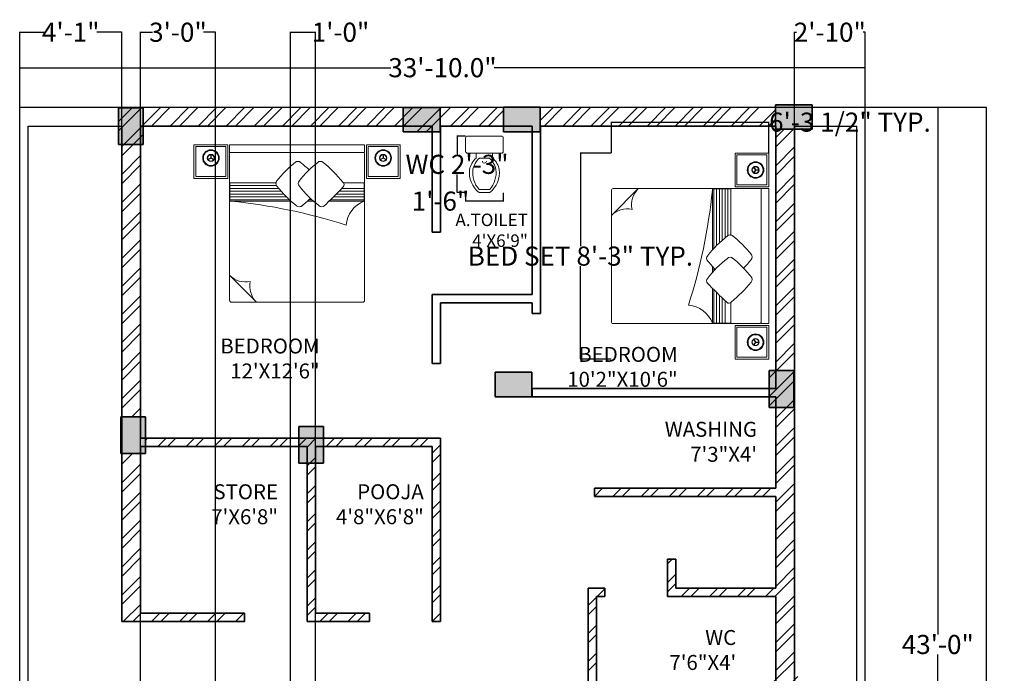
# Model space of a CAD drawing. Units: inches. Extents: x 104 to 629, y 1868 to 5138.
# Tile 2 of 2: x 156 to 629, y 2309 to 2623. Entities that reach past the tile are written whole.
import ezdxf

# ---------------------------------------------------------------- set-up
doc = ezdxf.new("R2010")
doc.units = ezdxf.units.IN
for name, color, linetype, lineweight in [('00 FURNITURE', 15, 'Continuous', 15), ('A-ANNO-DIMS', 2, 'Continuous', 18), ('A-AREA-IDEN', 7, 'Continuous', 18), ('A-FLOR-FIXT', 9, 'Continuous', 18), ('A-WALL-PATT', 8, 'Continuous', 13), ('C-PROP', 7, 'Continuous', 25), ('column', 10, 'Continuous', 35), ('hatch column', 10, 'Continuous', 13), ('WALL', 7, 'Continuous', 35)]:
    doc.layers.add(name, color=color, linetype=linetype, lineweight=lineweight)
doc.styles.get("Standard").update_dxf_attribs({"font": 'arial.ttf'})
doc.dimstyles.get("Standard").update_dxf_attribs({"dimtxt": 9.18, "dimasz": 0.18, "dimexe": 0.18, "dimexo": 0.0625, "dimgap": 0.09, "dimtad": 0, "dimtih": 1, "dimtoh": 1, "dimdec": 1, "dimzin": 0, "dimdsep": 46, "dimlunit": 3, "dimtxsty": 'Standard', "dimcen": 0.09, "dimadec": 0, "dimazin": 0, "dimtfac": 1, "dimtdec": 1, "dimtofl": 0, "dimtmove": 0, "dimatfit": 3, "dimfxl": 1, "dimtolj": 1, "dimtzin": 0, "dimarcsym": 0})

# ---------------------------------------------------------------- blocks, each defined once
blk = doc.blocks.new('column')
at = {"layer": 'column'}
for p, q in [((661.29, 2690.99), (673.05, 2690.99)), ((661.29, 2673.35), (661.29, 2690.99)), ((673.05, 2690.99), (673.05, 2673.35)), ((673.05, 2673.35), (661.29, 2673.35))]:
    blk.add_line(p, q, dxfattribs=at)
blk = doc.blocks.new('RGWTG')
at = {"layer": '00 FURNITURE'}
for p, q in [((578.23, 3473.51), (577.36, 3475.01)), ((578.36, 3473.58), (577.49, 3475.09)), ((578.23, 3473.58), (577.36, 3472.08)), ((578.36, 3473.51), (577.49, 3472)), ((578.29, 3473.62), (580.03, 3473.62)), ((578.29, 3473.47), (580.03, 3473.47)), ((521.93, 3464.58), (509.03, 3451.68)), ((509.03, 3422.63), (509.03, 3463.68)), ((509.93, 3464.58), (566.4, 3464.58)), ((557.53, 3463.84), (557.53, 3464.49)), ((557.53, 3464.49), (566.4, 3464.49)), ((558.2, 3464.49), (558.2, 3435.82)), ((559.57, 3464.49), (559.57, 3437.25)), ((560.94, 3464.49), (560.94, 3438.58)), ((562.3, 3464.49), (562.3, 3439.83)), ((563.67, 3464.49), (563.67, 3440.99)), ((565.04, 3464.49), (565.04, 3442.08)), ((566.4, 3464.58), (580.98, 3464.58)), ((566.4, 3464.49), (566.4, 3442.08)), ((566.4, 3464.49), (566.4, 3463.84)), ((580.98, 3464.58), (580.98, 3416.72)), ((558.2, 3426.48), (558.2, 3425.04)), ((509.03, 3400.68), (509.03, 3422.63)), ((558.2, 3416.13), (558.2, 3399.95)), ((559.57, 3414.75), (559.57, 3399.95)), ((580.98, 3416.72), (580.98, 3400.68)), ((560.94, 3413.39), (560.94, 3399.95)), ((562.3, 3412.04), (562.3, 3399.95)), ((563.67, 3410.72), (563.67, 3399.95)), ((580.08, 3399.78), (509.93, 3399.78)), ((557.53, 3399.95), (557.53, 3400.6)), ((566.4, 3399.95), (557.53, 3399.95)), ((566.4, 3400.6), (566.4, 3399.95)), ((578.23, 3390.78), (577.36, 3392.29)), ((578.23, 3390.86), (577.36, 3389.36)), ((578.36, 3390.86), (577.49, 3392.36)), ((578.36, 3390.78), (577.49, 3389.28)), ((578.29, 3390.9), (580.03, 3390.9)), ((578.29, 3390.74), (580.03, 3390.74))]:
    blk.add_line(p, q, dxfattribs=at)
for points in [[(568.43, 3465.48), (584.63, 3465.48), (584.63, 3481.68), (568.43, 3481.68)], [(569.33, 3466.38), (583.73, 3466.38), (583.73, 3480.78), (569.33, 3480.78)], [(580.98, 3399.78), (584.63, 3399.78), (584.63, 3464.58), (580.98, 3464.58)], [(568.43, 3398.88), (584.63, 3398.88), (584.63, 3382.68), (568.43, 3382.68)], [(569.33, 3397.98), (583.73, 3397.98), (583.73, 3383.58), (569.33, 3383.58)]]:
    blk.add_lwpolyline(points, close=True, dxfattribs=at)
for points in [[(566.52, 3464.49), (557.53, 3464.49), (557.53, 3435.08)], [(557.53, 3427.21), (557.53, 3424.3)], [(557.53, 3416.82), (557.53, 3399.95), (566.4, 3399.95), (566.4, 3409.94)]]:
    blk.add_lwpolyline(points, dxfattribs=at)
for centre, radius in [((578.29, 3473.54), 3.97), ((578.29, 3473.54), 3.63), ((578.29, 3473.54), 1.74), ((578.29, 3473.54), 1.56), ((578.29, 3390.82), 3.97), ((578.29, 3390.82), 3.63), ((578.29, 3390.82), 1.74), ((578.29, 3390.82), 1.56)]:
    blk.add_circle(centre, radius, dxfattribs=at)
for centre, radius, start, end in [((509.93, 3463.68), 0.9, 90, 180), ((529.65, 3456.88), 10.9, 135.0361, 191.9278), ((290.56, 3490.52), 268.3, 342.2214, 354.2925), ((516.73, 3443.97), 10.9, 78.0722, 134.9639), ((566.05, 3440.57), 1.82, 45, 135), ((533.58, 3399.31), 54.32, 37.931, 52.069), ((598.15, 3399.01), 54.32, 127.931, 142.069), ((574.84, 3431.77), 1.82, 315, 45), ((556.59, 3431.11), 1.82, 135, 225), ((597.87, 3463.6), 54.32, 217.931, 224.141), ((598.15, 3388.23), 54.32, 127.931, 142.069), ((566.05, 3429.78), 1.82, 45, 135), ((533.58, 3388.53), 54.32, 37.931, 52.069), ((533.28, 3463.88), 54.32, 316.32, 322.069), ((556.59, 3420.33), 1.82, 135, 225), ((765.33, 3619.75), 290.45, 223.6069, 226.2326), ((533.28, 3453.1), 54.32, 307.931, 322.069), ((574.84, 3420.99), 1.82, 315, 45), ((565.44, 3411.05), 1.47, 225.9674, 326.8337), ((545.02, 3395.29), 13.35, 20.4224, 85.5825), ((509.93, 3400.68), 0.9, 180, 270), ((580.08, 3400.68), 0.9, 270, 0)]:
    blk.add_arc(centre, radius, start, end, dxfattribs=at)
blk = doc.blocks.new('A$C2AC94788')
for p, q in [((0, 0.505), (0, 0.665)), ((0.025, 0.69), (0.435, 0.69)), ((0.46, 0.665), (0.46, 0.505)), ((0.435, 0.48), (0.025, 0.48)), ((0.13, 0.48), (0.13, 0.42)), ((0.17, 0.42), (0.29, 0.42)), ((0.33, 0.42), (0.33, 0.48)), ((0.164, 0.039), (0.296, 0.039)), ((0.229, 0.039), (0.23, 0.039)), ((0.231, 0.039), (0.23, 0.039)), ((0.165, 0), (0.295, 0))]:
    blk.add_line(p, q)
for centre, radius, start, end in [((0.025, 0.665), 0.025, 90, 180), ((0.435, 0.665), 0.025, 0, 90), ((0.025, 0.505), 0.025, 180, 270), ((0.435, 0.505), 0.025, 270, 0), ((0.287, 0.236), 0.242, 130.4885, 169.445), ((0.327, 0.236), 0.242, 130.4885, 169.445), ((0.23, 0.385), 0.025, 180, 0), ((0.133, 0.236), 0.242, 10.555, 49.5115), ((0.173, 0.236), 0.242, 10.555, 49.5115), ((0.36, 0.245), 0.313, 173.5369, 231.4483), ((0.4, 0.245), 0.313, 173.5369, 221.0604), ((0.1, 0.245), 0.313, 308.5517, 6.4631), ((0.06, 0.245), 0.313, 318.9396, 6.4631)]:
    blk.add_arc(centre, radius, start, end)
blk = doc.blocks.new('*D13')
at = {"layer": 'A-ANNO-DIMS', "color": 0, "lineweight": -2, "transparency": 16777216}
for p, q in [((155.91, 2581.05), (155.91, 2600.18)), ((156.09, 2600), (334.14, 2600)), ((561.73, 2600), (383.68, 2600)), ((561.91, 2581.05), (561.91, 2600.18))]:
    blk.add_line(p, q, dxfattribs=at)
at = {"layer": 'A-ANNO-DIMS', "color": 0, "transparency": 16777216}
for points in [[(156.09, 2600.03), (156.09, 2599.97), (155.91, 2600)], [(561.73, 2600.03), (561.73, 2599.97), (561.91, 2600)]]:
    blk.add_solid(points, dxfattribs=at)
at = {"layer": 'Defpoints', "color": 0, "transparency": 16777216}
for p in [(561.91, 2600), (155.91, 2580.99), (561.91, 2580.99)]:
    blk.add_point(p, dxfattribs=at)
at = {"layer": 'A-ANNO-DIMS', "color": 0, "transparency": 16777216, "insert": (358.91, 2600), "char_height": 9.18, "attachment_point": 5}
blk.add_mtext('\\A1;33\'-10.0"', dxfattribs=at)
blk = doc.blocks.new('*D14')
at = {"layer": 'A-ANNO-DIMS', "color": 0, "lineweight": -2, "transparency": 16777216}
for p, q in [((561.97, 2580.99), (620.18, 2580.99)), ((620, 2580.81), (620, 2249.77)), ((620, 1909.17), (620, 2240.21)), ((561.97, 1908.99), (620.18, 1908.99))]:
    blk.add_line(p, q, dxfattribs=at)
at = {"layer": 'A-ANNO-DIMS', "color": 0, "transparency": 16777216}
for points in [[(619.97, 2580.81), (620.03, 2580.81), (620, 2580.99)], [(619.97, 1909.17), (620.03, 1909.17), (620, 1908.99)]]:
    blk.add_solid(points, dxfattribs=at)
at = {"layer": 'Defpoints', "color": 0, "transparency": 16777216}
for p in [(561.91, 2580.99), (561.91, 1908.99), (620, 1908.99)]:
    blk.add_point(p, dxfattribs=at)
at = {"layer": 'A-ANNO-DIMS', "color": 0, "transparency": 16777216, "insert": (620, 2244.99), "char_height": 9.18, "attachment_point": 5}
blk.add_mtext("\\A1;56'", dxfattribs=at)
blk = doc.blocks.new('*D17')
at = {"layer": 'A-ANNO-DIMS', "color": 0, "lineweight": -2, "transparency": 16777216}
for p, q in [((439.94, 2559), (424.97, 2559)), ((425.15, 2558.82), (425.15, 2514.34)), ((425.15, 2460.18), (425.15, 2504.66)), ((439.94, 2460), (424.97, 2460))]:
    blk.add_line(p, q, dxfattribs=at)
at = {"layer": 'A-ANNO-DIMS', "color": 0, "transparency": 16777216}
for points in [[(425.12, 2558.82), (425.18, 2558.82), (425.15, 2559)], [(425.12, 2460.18), (425.18, 2460.18), (425.15, 2460)]]:
    blk.add_solid(points, dxfattribs=at)
at = {"layer": 'Defpoints', "color": 0, "transparency": 16777216}
for p in [(425.15, 2559), (440, 2559), (440, 2460)]:
    blk.add_point(p, dxfattribs=at)
at = {"layer": 'A-ANNO-DIMS', "color": 0, "transparency": 16777216, "insert": (425.15, 2509.5), "char_height": 9.18, "attachment_point": 5}
blk.add_mtext('\\A1;BED SET 8\'-3" TYP.', dxfattribs=at)
blk = doc.blocks.new('*D18')
at = {"layer": 'A-ANNO-DIMS', "color": 0, "lineweight": -2, "transparency": 16777216}
for p, q in [((440, 2559.06), (440, 2574.03)), ((440.18, 2573.85), (515.42, 2573.85)), ((515.6, 2559.06), (515.6, 2574.03)), ((515.6, 2573.85), (515.78, 2573.85))]:
    blk.add_line(p, q, dxfattribs=at)
at = {"layer": 'A-ANNO-DIMS', "color": 0, "transparency": 16777216}
for points in [[(440.18, 2573.88), (440.18, 2573.82), (440, 2573.85)], [(515.42, 2573.88), (515.42, 2573.82), (515.6, 2573.85)]]:
    blk.add_solid(points, dxfattribs=at)
at = {"layer": 'Defpoints', "color": 0, "transparency": 16777216}
for p in [(515.6, 2573.85), (440, 2559), (515.6, 2559)]:
    blk.add_point(p, dxfattribs=at)
at = {"layer": 'A-ANNO-DIMS', "color": 0, "transparency": 16777216, "insert": (554.57, 2573.85), "char_height": 9.18, "attachment_point": 5}
blk.add_mtext('\\A1;6\'-3 1/2" TYP.', dxfattribs=at)
blk = doc.blocks.new('*D23')
at = {"layer": 'A-ANNO-DIMS', "color": 0, "lineweight": -2, "transparency": 16777216}
for p, q in [((369.94, 2567.17), (365.74, 2567.17)), ((365.92, 2566.99), (365.92, 2558.42)), ((365.92, 2540.18), (365.92, 2548.74)), ((369.94, 2540), (365.74, 2540))]:
    blk.add_line(p, q, dxfattribs=at)
at = {"layer": 'A-ANNO-DIMS', "color": 0, "transparency": 16777216}
for points in [[(365.89, 2566.99), (365.95, 2566.99), (365.92, 2567.17)], [(365.89, 2540.18), (365.95, 2540.18), (365.92, 2540)]]:
    blk.add_solid(points, dxfattribs=at)
at = {"layer": 'Defpoints', "color": 0, "transparency": 16777216}
for p in [(365.92, 2567.17), (370, 2567.17), (370, 2540)]:
    blk.add_point(p, dxfattribs=at)
at = {"layer": 'A-ANNO-DIMS', "color": 0, "transparency": 16777216, "insert": (365.92, 2553.58), "char_height": 9.18, "attachment_point": 5}
blk.add_mtext('\\A1;WC 2\'-3"', dxfattribs=at)
blk = doc.blocks.new('*D24')
at = {"layer": 'A-ANNO-DIMS', "color": 0, "lineweight": -2, "transparency": 16777216}
for p, q in [((370, 2539.94), (370, 2535.74)), ((388.11, 2539.94), (388.11, 2535.74)), ((370, 2535.92), (369.82, 2535.92)), ((387.93, 2535.92), (370.18, 2535.92))]:
    blk.add_line(p, q, dxfattribs=at)
at = {"layer": 'A-ANNO-DIMS', "color": 0, "transparency": 16777216}
for points in [[(370.18, 2535.95), (370.18, 2535.89), (370, 2535.92)], [(387.93, 2535.95), (387.93, 2535.89), (388.11, 2535.92)]]:
    blk.add_solid(points, dxfattribs=at)
at = {"layer": 'Defpoints', "color": 0, "transparency": 16777216}
for p in [(370, 2540), (388.11, 2540), (370, 2535.92)]:
    blk.add_point(p, dxfattribs=at)
at = {"layer": 'A-ANNO-DIMS', "color": 0, "transparency": 16777216, "insert": (357.96, 2535.92), "char_height": 9.18, "attachment_point": 5}
blk.add_mtext('\\A1;1\'-6"', dxfattribs=at)
blk = doc.blocks.new('*D25')
at = {"layer": 'A-ANNO-DIMS', "color": 0, "lineweight": -2, "transparency": 16777216}
for p, q in [((155.91, 2581.05), (155.91, 2617.21)), ((156.09, 2617.03), (167.93, 2617.03)), ((204.73, 2617.03), (192.88, 2617.03)), ((204.91, 2572.05), (204.91, 2617.21))]:
    blk.add_line(p, q, dxfattribs=at)
at = {"layer": 'A-ANNO-DIMS', "color": 0, "transparency": 16777216}
for points in [[(156.09, 2617.06), (156.09, 2617), (155.91, 2617.03)], [(204.73, 2617.06), (204.73, 2617), (204.91, 2617.03)]]:
    blk.add_solid(points, dxfattribs=at)
at = {"layer": 'Defpoints', "color": 0, "transparency": 16777216}
for p in [(204.91, 2617.03), (155.91, 2580.99), (204.91, 2571.99)]:
    blk.add_point(p, dxfattribs=at)
at = {"layer": 'A-ANNO-DIMS', "color": 0, "transparency": 16777216, "insert": (180.41, 2617.03), "char_height": 9.18, "attachment_point": 5}
blk.add_mtext('\\A1;4\'-1"', dxfattribs=at)
blk = doc.blocks.new('*D26')
at = {"layer": 'A-ANNO-DIMS', "color": 0, "lineweight": -2, "transparency": 16777216}
for p, q in [((527.91, 2572.05), (527.91, 2617.21)), ((528.09, 2617.03), (528.97, 2617.03)), ((561.73, 2617.03), (560.84, 2617.03)), ((561.91, 2581.05), (561.91, 2617.21))]:
    blk.add_line(p, q, dxfattribs=at)
at = {"layer": 'A-ANNO-DIMS', "color": 0, "transparency": 16777216}
for points in [[(528.09, 2617.06), (528.09, 2617), (527.91, 2617.03)], [(561.73, 2617.06), (561.73, 2617), (561.91, 2617.03)]]:
    blk.add_solid(points, dxfattribs=at)
at = {"layer": 'Defpoints', "color": 0, "transparency": 16777216}
for p in [(561.91, 2617.03), (561.91, 2580.99), (527.91, 2571.99)]:
    blk.add_point(p, dxfattribs=at)
at = {"layer": 'A-ANNO-DIMS', "color": 0, "transparency": 16777216, "insert": (544.91, 2617.03), "char_height": 9.18, "attachment_point": 5}
blk.add_mtext('\\A1;2\'-10"', dxfattribs=at)
blk = doc.blocks.new('*D27')
at = {"layer": 'A-ANNO-DIMS', "color": 0, "lineweight": -2, "transparency": 16777216}
for p, q in [((405.93, 2580.97), (596.94, 2580.97)), ((596.76, 2580.79), (596.76, 2327.76)), ((596.76, 2065.18), (596.76, 2318.2)), ((527.99, 2065), (596.94, 2065))]:
    blk.add_line(p, q, dxfattribs=at)
at = {"layer": 'A-ANNO-DIMS', "color": 0, "transparency": 16777216}
for points in [[(596.73, 2580.79), (596.79, 2580.79), (596.76, 2580.97)], [(596.73, 2065.18), (596.79, 2065.18), (596.76, 2065)]]:
    blk.add_solid(points, dxfattribs=at)
at = {"layer": 'Defpoints', "color": 0, "transparency": 16777216}
for p in [(405.87, 2580.97), (596.76, 2580.97), (527.93, 2065)]:
    blk.add_point(p, dxfattribs=at)
at = {"layer": 'A-ANNO-DIMS', "color": 0, "transparency": 16777216, "insert": (596.76, 2322.98), "char_height": 9.18, "attachment_point": 5}
blk.add_mtext('\\A1;43\'-0"', dxfattribs=at)
blk = doc.blocks.new('*D31')
at = {"layer": 'A-ANNO-DIMS', "color": 0, "lineweight": -2, "transparency": 16777216}
for p, q in [((213.91, 2074.05), (213.91, 2617.21)), ((214.09, 2617.03), (219.62, 2617.03)), ((249.73, 2617.03), (244.2, 2617.03)), ((249.91, 2074.05), (249.91, 2617.21))]:
    blk.add_line(p, q, dxfattribs=at)
at = {"layer": 'A-ANNO-DIMS', "color": 0, "transparency": 16777216}
for points in [[(214.09, 2617.06), (214.09, 2617), (213.91, 2617.03)], [(249.73, 2617.06), (249.73, 2617), (249.91, 2617.03)]]:
    blk.add_solid(points, dxfattribs=at)
at = {"layer": 'Defpoints', "color": 0, "transparency": 16777216}
for p in [(249.91, 2617.03), (213.91, 2073.99), (249.91, 2073.99)]:
    blk.add_point(p, dxfattribs=at)
at = {"layer": 'A-ANNO-DIMS', "color": 0, "transparency": 16777216, "insert": (231.91, 2617.03), "char_height": 9.18, "attachment_point": 5}
blk.add_mtext('\\A1;3\'-0"', dxfattribs=at)
blk = doc.blocks.new('*D36')
at = {"layer": 'A-ANNO-DIMS', "color": 0, "lineweight": -2, "transparency": 16777216}
for p, q in [((285.91, 2166.05), (285.91, 2617.21)), ((286.09, 2617.03), (297.73, 2617.03)), ((297.91, 2166.05), (297.91, 2617.21)), ((297.91, 2617.03), (298.09, 2617.03))]:
    blk.add_line(p, q, dxfattribs=at)
at = {"layer": 'A-ANNO-DIMS', "color": 0, "transparency": 16777216}
for points in [[(286.09, 2617.06), (286.09, 2617), (285.91, 2617.03)], [(297.73, 2617.06), (297.73, 2617), (297.91, 2617.03)]]:
    blk.add_solid(points, dxfattribs=at)
at = {"layer": 'Defpoints', "color": 0, "transparency": 16777216}
for p in [(297.91, 2617.03), (285.91, 2165.99), (297.91, 2165.99)]:
    blk.add_point(p, dxfattribs=at)
at = {"layer": 'A-ANNO-DIMS', "color": 0, "transparency": 16777216, "insert": (309.95, 2617.03), "char_height": 9.18, "attachment_point": 5}
blk.add_mtext('\\A1;1\'-0"', dxfattribs=at)

msp = doc.modelspace()

# ---------------------------------------------------------------- hatches: boundary and pattern name
at = {"layer": 'A-WALL-PATT'}
h = msp.add_hatch(dxfattribs=at)
h.set_pattern_fill('ANSI32', color=256)
h.paths.add_polyline_path([(518.75, 2580.99), (405.87, 2580.99), (405.87, 2571.99), (518.75, 2571.99)])
h.paths.add_polyline_path([(357.74, 2580.99), (357.74, 2569.19), (340.1, 2569.19), (340.1, 2571.99), (215.15, 2571.99), (215.15, 2563.15), (203.39, 2563.15), (203.39, 2580.99)])
h.paths.add_polyline_path([(388.23, 2580.99), (357.74, 2580.99), (357.74, 2571.99), (388.23, 2571.99)])
h.paths.add_polyline_path([(213.91, 2563.15), (204.91, 2563.15), (204.91, 2432.29), (213.91, 2432.29)])
h.paths.add_polyline_path([(527.91, 2570.42), (518.91, 2570.42), (518.91, 2454.51), (527.91, 2454.51)])
h.paths.add_polyline_path([(213.91, 2414.65), (204.91, 2414.65), (204.91, 2333.99), (263.91, 2333.99), (263.91, 2337.99), (213.91, 2337.99)])
h.paths.add_polyline_path([(290, 2421.99), (216.27, 2421.99), (216.27, 2417.99), (290, 2417.99)])
h.paths.add_polyline_path([(357.91, 2421.99), (290, 2421.99), (290, 2417.99), (293.91, 2417.99), (293.91, 2333.99), (323.91, 2333.99), (323.91, 2337.99), (297.91, 2337.99), (297.91, 2417.99), (353.91, 2417.99), (353.91, 2333.99), (357.91, 2333.99)])
h = msp.add_hatch(dxfattribs=at)
h.set_pattern_fill('ANSI32', color=256)
h.paths.add_polyline_path([(527.91, 2307.64), (530, 2307.64), (530, 2290), (518.24, 2290), (518.24, 2307.64), (518.91, 2307.64), (518.91, 2345.99), (466.91, 2345.99), (466.91, 2363.99), (470.91, 2363.99), (470.91, 2349.99), (518.91, 2349.99), (518.91, 2393.99), (431.91, 2393.99), (431.91, 2397.99), (518.91, 2397.99), (518.91, 2436.87), (515.84, 2436.87), (515.84, 2454.51), (527.91, 2454.51)])
h.paths.add_polyline_path([(432.91, 2345.99), (436.91, 2345.99), (436.91, 2349.99), (428.91, 2349.99), (428.91, 2297.99), (411.76, 2297.99), (411.76, 2293.99), (518.24, 2293.99), (518.24, 2297.99), (432.91, 2297.99)])
at = {"layer": 'hatch column', "transparency": 33554559}
h = msp.add_hatch(color=256, dxfattribs=at)
h.dxf.hatch_style = 1
h.paths.add_polyline_path([(518.75, 2582.18), (518.75, 2570.42), (536.39, 2570.42), (536.39, 2582.18)])
h = msp.add_hatch(color=256, dxfattribs=at)
h.dxf.hatch_style = 1
h.paths.add_polyline_path([(203.39, 2563.15), (215.15, 2563.15), (215.15, 2580.79), (203.39, 2580.79)])
h = msp.add_hatch(color=256, dxfattribs=at)
h.dxf.hatch_style = 1
h.paths.add_polyline_path([(357.74, 2569.19), (357.74, 2580.95), (340.1, 2580.95), (340.1, 2569.19)])
h = msp.add_hatch(color=256, dxfattribs=at)
h.dxf.hatch_style = 1
h.paths.add_polyline_path([(405.87, 2569.21), (405.87, 2580.97), (388.23, 2580.97), (388.23, 2569.21)])
h = msp.add_hatch(color=256, dxfattribs=at)
h.dxf.hatch_style = 1
h.paths.add_polyline_path([(384.27, 2453.75), (384.27, 2441.99), (401.91, 2441.99), (401.91, 2453.75)])
h = msp.add_hatch(color=256, dxfattribs=at)
h.dxf.hatch_style = 1
h.paths.add_polyline_path([(527.6, 2436.87), (527.6, 2454.51), (515.84, 2454.51), (515.84, 2436.87)])
h = msp.add_hatch(color=256, dxfattribs=at)
h.dxf.hatch_style = 1
h.paths.add_polyline_path([(204.51, 2414.65), (216.27, 2414.65), (216.27, 2432.29), (204.51, 2432.29)])
h = msp.add_hatch(color=256, dxfattribs=at)
h.dxf.hatch_style = 1
h.paths.add_polyline_path([(301.76, 2427.64), (290, 2427.64), (290, 2410), (301.76, 2410)])

# ---------------------------------------------------------------- linework, layer by layer
at = {"layer": 'C-PROP'}
for p, q in [((155.91, 2580.99), (561.91, 2580.99)), ((155.91, 1908.99), (155.91, 2580.99)), ((561.91, 1908.99), (561.91, 2580.99)), ((159.91, 1917.99), (159.91, 2571.99)), ((159.91, 2571.99), (204.91, 2571.99)), ((527.91, 2571.99), (557.91, 2571.99)), ((557.91, 1917.99), (557.91, 2571.99))]:
    msp.add_line(p, q, dxfattribs=at)
at = {"layer": 'WALL'}
for p, q in [((204.91, 2333.99), (204.91, 2571.99)), ((213.91, 2421.99), (213.91, 2571.99)), ((213.91, 2571.99), (353.91, 2571.99)), ((353.91, 2520.99), (353.91, 2571.99)), ((357.91, 2571.99), (401.91, 2571.99)), ((357.91, 2520.99), (357.91, 2571.99)), ((401.91, 2490.99), (401.91, 2571.99)), ((405.91, 2571.99), (518.91, 2571.99)), ((405.91, 2481.99), (405.91, 2571.99)), ((518.91, 2445.99), (518.91, 2571.99)), ((527.91, 2008.99), (527.91, 2571.99)), ((353.91, 2520.99), (357.91, 2520.99)), ((353.91, 2490.99), (401.91, 2490.99)), ((353.91, 2457.99), (353.91, 2490.99)), ((357.91, 2486.99), (401.91, 2486.99)), ((357.91, 2457.99), (357.91, 2486.99)), ((401.91, 2481.99), (401.91, 2486.99)), ((401.91, 2481.99), (405.91, 2481.99)), ((353.91, 2457.99), (357.91, 2457.99)), ((401.91, 2445.99), (518.91, 2445.99)), ((401.91, 2441.99), (401.91, 2445.99)), ((401.91, 2441.99), (518.91, 2441.99)), ((518.91, 2397.99), (518.91, 2441.99)), ((213.91, 2421.99), (357.91, 2421.99)), ((357.91, 2333.99), (357.91, 2421.99)), ((213.91, 2417.99), (293.91, 2417.99)), ((213.91, 2337.99), (213.91, 2417.99)), ((293.91, 2333.99), (293.91, 2417.99)), ((297.91, 2337.99), (297.91, 2417.99)), ((297.91, 2417.99), (353.91, 2417.99)), ((353.91, 2337.99), (353.91, 2417.99)), ((353.91, 2333.99), (353.91, 2417.99)), ((431.91, 2397.99), (518.91, 2397.99)), ((431.91, 2393.99), (431.91, 2397.99)), ((431.91, 2393.99), (518.91, 2393.99)), ((518.91, 2349.99), (518.91, 2393.99)), ((466.91, 2345.99), (466.91, 2363.99)), ((466.91, 2363.99), (470.91, 2363.99)), ((470.91, 2349.99), (470.91, 2363.99)), ((428.91, 2349.99), (436.91, 2349.99)), ((428.91, 2297.99), (428.91, 2349.99)), ((436.91, 2345.99), (436.91, 2349.99)), ((470.91, 2349.99), (518.91, 2349.99)), ((432.91, 2345.99), (436.91, 2345.99)), ((432.91, 2297.99), (432.91, 2345.99)), ((466.91, 2345.99), (518.91, 2345.99)), ((518.91, 2297.99), (518.91, 2345.99)), ((213.91, 2337.99), (263.91, 2337.99)), ((263.91, 2333.99), (263.91, 2337.99)), ((297.91, 2337.99), (323.91, 2337.99)), ((323.91, 2333.99), (323.91, 2337.99)), ((204.91, 2333.99), (263.91, 2333.99)), ((293.91, 2333.99), (323.91, 2333.99)), ((353.91, 2333.99), (357.91, 2333.99))]:
    msp.add_line(p, q, dxfattribs=at)

# ---------------------------------------------------------------- block references
at = {"layer": '00 FURNITURE', "rotation": 89.99999999999999}
msp.add_blockref('RGWTG', (3721.28, 1978.35), dxfattribs=at)
at = {"layer": '00 FURNITURE'}
msp.add_blockref('RGWTG', (-69.03, -922.68), dxfattribs=at)
at = {"layer": 'A-FLOR-FIXT', "xscale": -39.375, "yscale": 39.375, "zscale": 39.375}
msp.add_blockref('A$C2AC94788', (388.11, 2540), dxfattribs=at)
at = {"layer": 'column'}
for p, rotation in [((-2154.6, 3243.47), 270), ((-2333.26, 3242.24), 270), ((-2285.12, 3242.26), 270), ((-2289.09, 3115.04), 270.0000012926876)]:
    msp.add_blockref('column', p, dxfattribs=dict(at, rotation=rotation))
for p in [(-457.9, -110.2), (-145.45, -236.49), (-456.79, -258.71), (-371.29, -263.35)]:
    msp.add_blockref('column', p, dxfattribs=at)

# ---------------------------------------------------------------- texts
at = {"layer": 'A-AREA-IDEN', "attachment_point": 3}
for s, insert, char_height in [(' {\\H0.83478x;A.TOILET 4\'X6\'9"}', (399.94, 2529.92), 7.1875), ('BEDROOM\\P12\'X12\'6"', (299.94, 2469.92), 7.188), ('BEDROOM\\P10\'2"X10\'6"', (471.85, 2465.91), 7.1875), ('WASHING\\P7\'3"X4\'', (509.94, 2429.92), 7.188), ('STORE\\P7\'X6\'8"', (279.94, 2399.92), 7.188), ('POOJA\\P4\'8"X6\'8"', (349.94, 2399.92), 7.188), ('WC\\P7\'6"X4\'', (499.94, 2329.92), 7.188)]:
    msp.add_mtext_dynamic_manual_height_columns(s, width=41.3807, gutter_width=12.5, heights=[0], dxfattribs=dict(at, insert=insert, char_height=char_height))

# ---------------------------------------------------------------- dimensions: what is measured, and where the dimension line sits
at = {"layer": 'A-ANNO-DIMS'}
for base, p1, p2, override, picture, middle in [((204.91, 2617.03), (155.91, 2580.99), (204.91, 2571.99), {"dimdec": 1, "dimlfac": 1, "dimrnd": 0, "dimzin": 1, "dimdsep": 46, "dimlunit": 4, "dimfrac": 2}, '*D25', (180.41, 2617.03)), ((249.91, 2617.03), (213.91, 2073.99), (249.91, 2073.99), {"dimdec": 1, "dimlfac": 1, "dimrnd": 0, "dimzin": 1, "dimdsep": 46, "dimlunit": 4, "dimfrac": 2}, '*D31', (231.91, 2617.03)), ((297.91, 2617.03), (285.91, 2165.99), (297.91, 2165.99), {"dimdec": 1, "dimlfac": 1, "dimrnd": 0, "dimzin": 1, "dimdsep": 46, "dimlunit": 4, "dimfrac": 2}, '*D36', (309.95, 2617.03)), ((561.91, 2617.03), (527.91, 2571.99), (561.91, 2580.99), {"dimdec": 1, "dimlfac": 1, "dimrnd": 0, "dimzin": 1, "dimdsep": 46, "dimlunit": 4, "dimfrac": 2}, '*D26', (544.91, 2617.03)), ((561.91, 2600), (155.91, 2580.99), (561.91, 2580.99), {"dimclrd": 0, "dimclre": 0, "dimclrt": 0}, '*D13', (358.91, 2600))]:
    dim = msp.add_linear_dim(base=base, p1=p1, p2=p2, dimstyle='Standard', override=override, dxfattribs=at)
    dim.commit()
    dim.dimension.update_dxf_attribs({"geometry": picture, "text_midpoint": middle})
dim = msp.add_linear_dim(base=(515.6, 2573.85), p1=(440, 2559), p2=(515.6, 2559), text='<> TYP.', dimstyle='Standard', override={"dimdec": 1, "dimlfac": 1, "dimrnd": 0, "dimzin": 1, "dimdsep": 46, "dimlunit": 4, "dimfrac": 2}, dxfattribs=at)
dim.commit()
dim.dimension.update_dxf_attribs({"geometry": '*D18', "text_midpoint": (554.57, 2573.85)})
for base, p1, p2, angle, override, picture, middle in [((596.76, 2580.97), (527.93, 2065), (405.87, 2580.97), 90, {"dimdec": 1, "dimlfac": 1, "dimrnd": 0, "dimzin": 1, "dimdsep": 46, "dimlunit": 4, "dimfrac": 2}, '*D27', (596.76, 2322.98)), ((620, 1908.99), (561.91, 2580.99), (561.91, 1908.99), 90, {"dimclrd": 0, "dimclre": 0, "dimclrt": 0}, '*D14', (620, 2244.99)), ((370, 2535.92), (388.11, 2540), (370, 2540), 180, {"dimdec": 1, "dimlfac": 1, "dimrnd": 0, "dimzin": 1, "dimdsep": 46, "dimlunit": 4, "dimfrac": 2}, '*D24', (357.96, 2535.92))]:
    dim = msp.add_linear_dim(base=base, p1=p1, p2=p2, angle=angle, dimstyle='Standard', override=override, dxfattribs=at)
    dim.commit()
    dim.dimension.update_dxf_attribs({"geometry": picture, "text_midpoint": middle})
for base, p1, p2, text, picture, middle in [((365.92, 2567.17), (370, 2540), (370, 2567.17), 'WC <>', '*D23', (365.92, 2553.58)), ((425.15, 2559), (440, 2460), (440, 2559), 'BED SET <> TYP.', '*D17', (425.15, 2509.5))]:
    dim = msp.add_linear_dim(base=base, p1=p1, p2=p2, angle=90, text=text, dimstyle='Standard', override={"dimdec": 1, "dimlfac": 1, "dimrnd": 0, "dimzin": 1, "dimdsep": 46, "dimlunit": 4, "dimfrac": 2}, dxfattribs=at)
    dim.commit()
    dim.dimension.update_dxf_attribs({"geometry": picture, "text_midpoint": middle})

doc.saveas('drawing.dxf')
